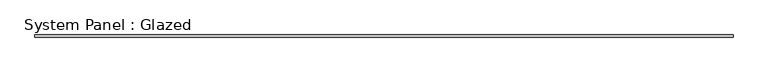
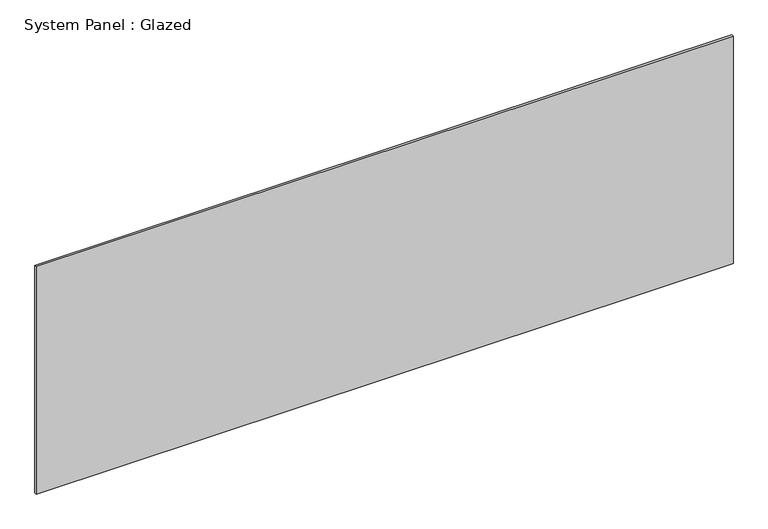
"""IFC4 building model written with IfcOpenShell, lengths in millimetres: plate geometry, System Panel : Glazed."""

from ifc_helpers import new_model, si_unit, origin, origin_with_axes, place, context, project, spatial, polyline, outline, extrude, source, transform, mapped, element, save


def system_panel_glazed_f36121af(model_context):
    return source(origin(), model_context, "Body", "SweptSolid", [
        extrude(outline(polyline([(4152.9174526, 19.05), (-4152.9174526, 19.05), (-4152.9174526, 44.45), (4152.9174526, 44.45), (4152.9174526, 19.05)])), origin_with_axes(), (0.0, 0.0, 1.0), 2867.5946513),
    ])


if __name__ == "__main__":
    model = new_model("IFC4")
    model_context = context("Model", 3, world=origin())
    ifc_project = project(units=[si_unit("LENGTHUNIT", "METRE", prefix="MILLI")], contexts=[model_context])
    site = spatial("IfcSite", under=ifc_project)
    building = spatial("IfcBuilding", under=site)
    placement = place(None, origin())
    system_panel_glazed_shape = system_panel_glazed_f36121af(model_context)
    element("IfcPlate", 1, ObjectType="System Panel : Glazed", at=placement, inside=building, context=model_context, shape_type="MappedRepresentation", body=[
        mapped(system_panel_glazed_shape, transform((0.0, 0.0, 0.0), x_axis=(1.0, 0.0, 0.0), y_axis=(0.0, 1.0, 0.0), z_axis=(0.0, 0.0, 1.0))),
    ])
    save(model, "model.ifc")

# Revit data of these elements
# Type "System Panel : Glazed"
#   Construction Type Id = "GSP4R"
#   Analytic Construction = "1/8 in Pilkington single glazing"
#   Visual Light Transmittance = 0.9
#   Solar Heat Gain Coefficient = 0.86
#   Heat Transfer Coefficient (U) = 1.18115 BTU/(h·ft²·°F)
#   Define Thermal Properties by = 1
# Element 1 (IfcPlate, "System Panel : Glazed")
#   Materials on its faces: "Glass"
# Materials
#   "Glass": class "Glass", colour RGB 0 128 192, transparency 0.75, Description = "Soda Lime Glass", Cost = 0
